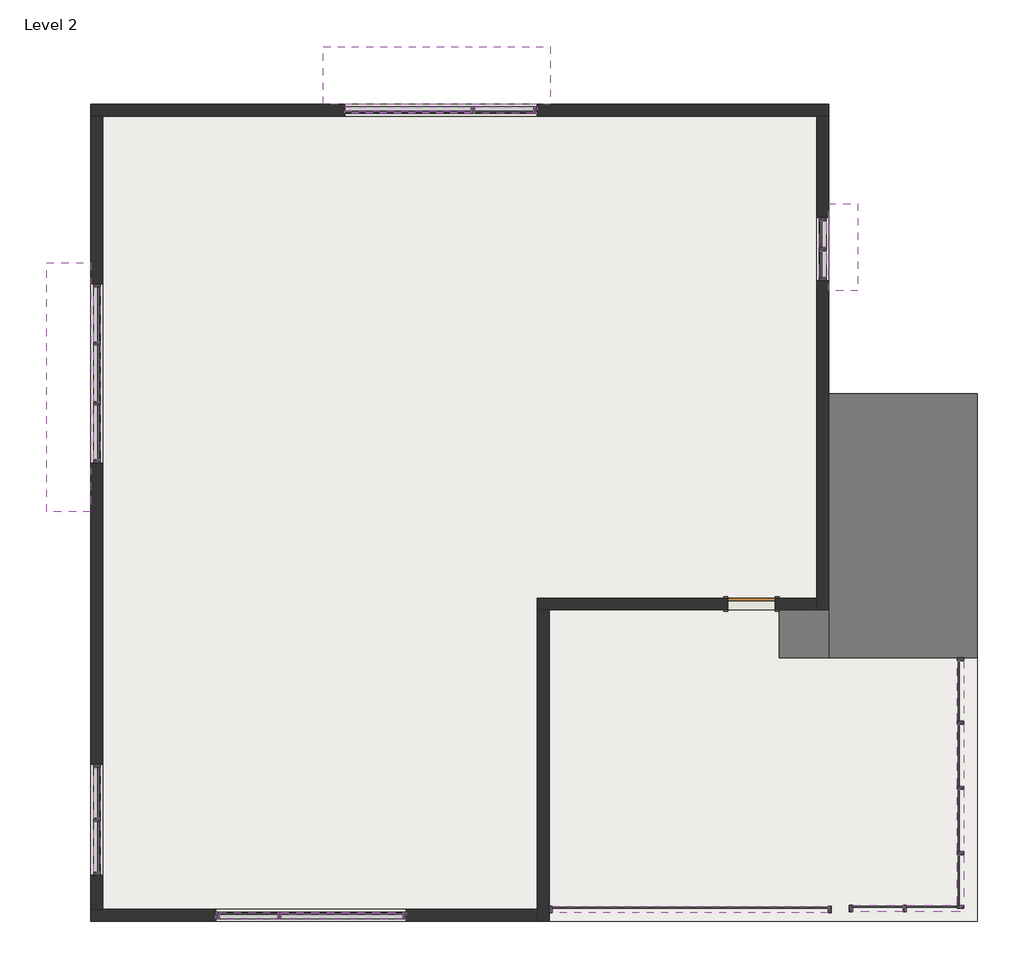
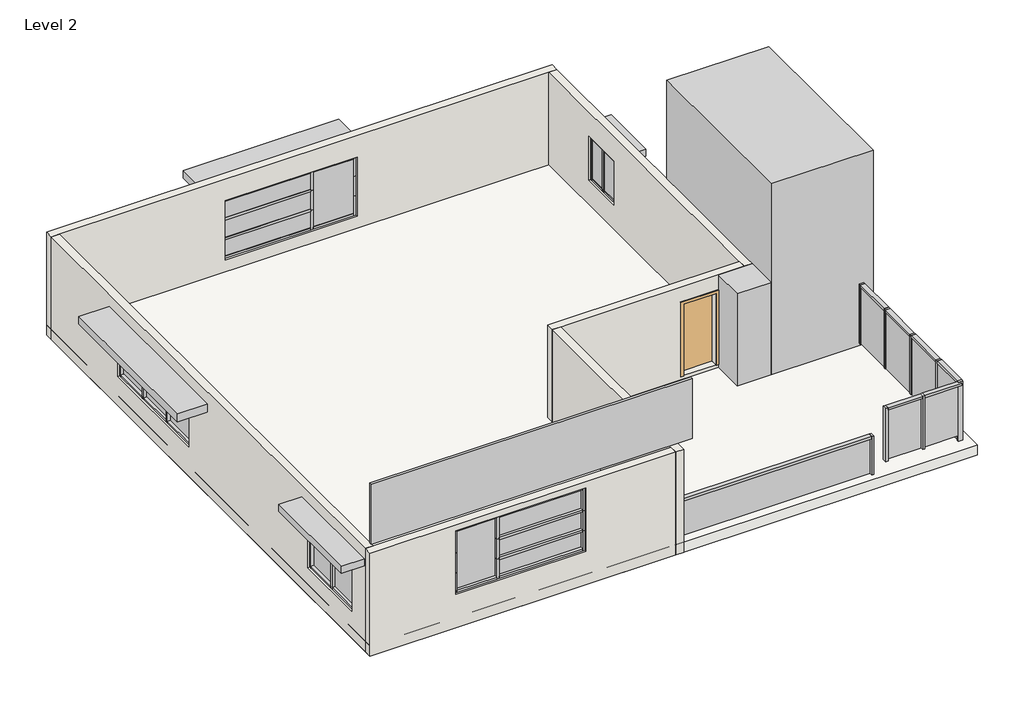
# One storey: 67 members, 22 plates, 6 walls, 4 proxies, 1 door, 1 roof.
"""IFC4 building model written with IfcOpenShell, lengths in millimetres."""

from ifc_helpers import new_model, si_unit, frame, origin, place, context, project, spatial, polyline, outline, extrude, faceted_brep, transform, mapped, element, save
from components import generic_models_10_generic_models_10_d4c633cf, generic_models_11_generic_models_11_9e8de572, generic_models_2_generic_models_2_10608999, generic_models_9_generic_models_9_222cebfa, door_0ca8825f, member_e6b9f524, member_eadc486f, member_9597caa3, member_f68a8c1e, member_c273ec95, member_b59b363a, member_48a7c542, member_a8f28920, member_ca95d35f, member_6d95fc69, member_971db604, member_6ef8dc49, member_801a2072, member_ed31d27a, member_2fbbe8c6, member_1434c356, member_89a24a7a, member_0b7646a3, member_9869c819, member_19a13f65, member_b030ebd8, member_54a35e60, member_39111128, member_6133cf7c, member_2569944f, member_814d5477, member_c450aece, member_9fa6ebbc, member_96c24052, member_491a8506, member_693a6220, system_panel_glazed_93d7cfd2, system_panel_glazed_c682d145, system_panel_glazed_b2f512c6, system_panel_glazed_6011e45a, system_panel_glazed_1356a548, system_panel_glazed_90125d95, system_panel_glazed_daa3f2c1, system_panel_glazed_8ae820b6, system_panel_glazed_a24099ce, system_panel_glazed_da159ad5, system_panel_glazed_d098f70f, system_panel_glazed_c8d94a63, system_panel_glazed_5b59eb94, system_panel_glazed_618c1181, system_panel_glazed_0e829309, system_panel_glazed_645b7f4f, system_panel_glazed_7de21dfc

model = new_model("IFC4")

# Units and contexts
model_context = context("Model", 3, world=origin())
ifc_project = project(units=[si_unit("LENGTHUNIT", "METRE", prefix="MILLI")], contexts=[model_context])

# Site, building, storey
site = spatial("IfcSite", under=ifc_project)
building = spatial("IfcBuilding", under=site)
storey = spatial("IfcBuildingStorey", under=building, Name="Level 2", Elevation=3048.0)

# Proxies
placement = place(None, origin())
generic_models_10_generic_models_10_shape = generic_models_10_generic_models_10_d4c633cf(model_context)
element("IfcBuildingElementProxy", 1, Name="Generic Models 10 : Generic Models 10", ObjectType="Generic Models 10 : Generic Models 10", at=placement, inside=storey, context=model_context, shape_type="MappedRepresentation", body=[
    mapped(generic_models_10_generic_models_10_shape, transform((0.0, 0.0, 0.0), x_axis=(1.0, 0.0, 0.0), y_axis=(0.0, 1.0, 0.0), z_axis=(0.0, 0.0, 1.0))),
])
generic_models_11_generic_models_11_shape = generic_models_11_generic_models_11_9e8de572(model_context)
element("IfcBuildingElementProxy", 2, Name="Generic Models 11 : Generic Models 11", ObjectType="Generic Models 11 : Generic Models 11", at=placement, inside=storey, context=model_context, shape_type="MappedRepresentation", body=[
    mapped(generic_models_11_generic_models_11_shape, transform((0.0, 0.0, 0.0), x_axis=(1.0, 0.0, 0.0), y_axis=(0.0, 1.0, 0.0), z_axis=(0.0, 0.0, 1.0))),
])
generic_models_2_generic_models_2_shape = generic_models_2_generic_models_2_10608999(model_context)
element("IfcBuildingElementProxy", 3, Name="Generic Models 2 : Generic Models 2", ObjectType="Generic Models 2 : Generic Models 2", at=placement, inside=storey, context=model_context, shape_type="MappedRepresentation", body=[
    mapped(generic_models_2_generic_models_2_shape, transform((0.0, 0.0, 0.0), x_axis=(1.0, 0.0, 0.0), y_axis=(0.0, 1.0, 0.0), z_axis=(0.0, 0.0, 1.0))),
])
generic_models_9_generic_models_9_shape = generic_models_9_generic_models_9_222cebfa(model_context)
element("IfcBuildingElementProxy", 4, Name="Generic Models 9 : Generic Models 9", ObjectType="Generic Models 9 : Generic Models 9", at=placement, inside=storey, context=model_context, shape_type="MappedRepresentation", body=[
    mapped(generic_models_9_generic_models_9_shape, transform((0.0, 0.0, 0.0), x_axis=(1.0, 0.0, 0.0), y_axis=(0.0, 1.0, 0.0), z_axis=(0.0, 0.0, 1.0))),
])

# Door
door_shape = door_0ca8825f(model_context)
element("IfcDoor", 5, ObjectType="Single-Flush : 36\" x 84\"", at=placement, inside=storey, context=model_context, shape_type="MappedRepresentation", body=[
    mapped(door_shape, transform((-7357.3120831, -6017.2945627, 3454.4), x_axis=(1.0, 0.0, 0.0), y_axis=(0.0, 1.0, 0.0), z_axis=(0.0, 0.0, 1.0))),
])

# Members
member_shape = member_e6b9f524(model_context)
element("IfcMember", 6, ObjectType="Rectangular Mullion : 2.5\" x 5\" rectangular", at=placement, inside=storey, context=model_context, shape_type="MappedRepresentation", body=[
    mapped(member_shape, transform((-16456.8620831, -11998.9945627, 5914.7350313), x_axis=(0.0, 0.0, 1.0), y_axis=(0.0, -1.0, 0.0), z_axis=(1.0, 0.0, 0.0))),
])
element("IfcMember", 7, ObjectType="Rectangular Mullion : 2.5\" x 5\" rectangular", at=placement, inside=storey, context=model_context, shape_type="MappedRepresentation", body=[
    mapped(member_shape, transform((-17580.8120831, -11998.9945627, 4036.0212725), x_axis=(0.0, 0.0, -1.0), y_axis=(0.0, -1.0, 0.0), z_axis=(-1.0, 0.0, 0.0))),
])
member_2_shape = member_eadc486f(model_context)
element("IfcMember", 8, ObjectType="Rectangular Mullion : 2.5\" x 5\" rectangular", at=placement, inside=storey, context=model_context, shape_type="MappedRepresentation", body=[
    mapped(member_2_shape, transform((-14050.2120831, -11998.9945627, 5914.7350313), x_axis=(0.0, 0.0, 1.0), y_axis=(0.0, -1.0, 0.0), z_axis=(1.0, 0.0, 0.0))),
])
element("IfcMember", 9, ObjectType="Rectangular Mullion : 2.5\" x 5\" rectangular", at=placement, inside=storey, context=model_context, shape_type="MappedRepresentation", body=[
    mapped(member_2_shape, transform((-16393.3620831, -11998.9945627, 4036.0212725), x_axis=(0.0, 0.0, -1.0), y_axis=(0.0, -1.0, 0.0), z_axis=(-1.0, 0.0, 0.0))),
])
member_3_shape = member_9597caa3(model_context)
element("IfcMember", 10, ObjectType="Rectangular Mullion : 2.5\" x 5\" rectangular", at=placement, inside=storey, context=model_context, shape_type="MappedRepresentation", body=[
    mapped(member_3_shape, transform((-14050.2120831, -11998.9945627, 5221.3329246), x_axis=(0.0, 0.0, 1.0), y_axis=(0.0, -1.0, 0.0), z_axis=(1.0, 0.0, 0.0))),
])
element("IfcMember", 11, ObjectType="Rectangular Mullion : 2.5\" x 5\" rectangular", at=placement, inside=storey, context=model_context, shape_type="MappedRepresentation", body=[
    mapped(member_3_shape, transform((-14050.2120831, -11998.9945627, 4628.6770985), x_axis=(0.0, 0.0, 1.0), y_axis=(0.0, -1.0, 0.0), z_axis=(1.0, 0.0, 0.0))),
])
member_4_shape = member_f68a8c1e(model_context)
element("IfcMember", 12, ObjectType="Rectangular Mullion : 2.5\" x 5\" rectangular", at=placement, inside=storey, context=model_context, shape_type="MappedRepresentation", body=[
    mapped(member_4_shape, transform((-17644.3120831, -11998.9945627, 5221.3329246), x_axis=(-1.0, 0.0, 0.0), y_axis=(0.0, -1.0, 0.0), z_axis=(0.0, 0.0, 1.0))),
])
element("IfcMember", 13, ObjectType="Rectangular Mullion : 2.5\" x 5\" rectangular", at=placement, inside=storey, context=model_context, shape_type="MappedRepresentation", body=[
    mapped(member_4_shape, transform((-17644.3120831, -11998.9945627, 4628.6770985), x_axis=(-1.0, 0.0, 0.0), y_axis=(0.0, -1.0, 0.0), z_axis=(0.0, 0.0, 1.0))),
])
member_5_shape = member_c273ec95(model_context)
element("IfcMember", 14, ObjectType="Rectangular Mullion : 2.5\" x 5\" rectangular", at=placement, inside=storey, context=model_context, shape_type="MappedRepresentation", body=[
    mapped(member_5_shape, transform((-16425.1120831, -11998.9945627, 4628.6770985), x_axis=(1.0, 0.0, 0.0), y_axis=(0.0, -1.0, 0.0), z_axis=(0.0, 0.0, -1.0))),
])
element("IfcMember", 15, ObjectType="Rectangular Mullion : 2.5\" x 5\" rectangular", at=placement, inside=storey, context=model_context, shape_type="MappedRepresentation", body=[
    mapped(member_5_shape, transform((-16425.1120831, -11998.9945627, 4036.0212725), x_axis=(1.0, 0.0, 0.0), y_axis=(0.0, -1.0, 0.0), z_axis=(0.0, 0.0, -1.0))),
])
element("IfcMember", 16, ObjectType="Rectangular Mullion : 2.5\" x 5\" rectangular", at=placement, inside=storey, context=model_context, shape_type="MappedRepresentation", body=[
    mapped(member_4_shape, transform((-13986.7120831, -11998.9945627, 4628.6770985), x_axis=(1.0, 0.0, 0.0), y_axis=(0.0, -1.0, 0.0), z_axis=(0.0, 0.0, -1.0))),
])
element("IfcMember", 17, ObjectType="Rectangular Mullion : 2.5\" x 5\" rectangular", at=placement, inside=storey, context=model_context, shape_type="MappedRepresentation", body=[
    mapped(member_4_shape, transform((-13986.7120831, -11998.9945627, 4036.0212725), x_axis=(1.0, 0.0, 0.0), y_axis=(0.0, -1.0, 0.0), z_axis=(0.0, 0.0, -1.0))),
])
member_6_shape = member_b59b363a(model_context)
element("IfcMember", 18, ObjectType="Rectangular Mullion : 2.5\" x 5\" rectangular", at=placement, inside=storey, context=model_context, shape_type="MappedRepresentation", body=[
    mapped(member_6_shape, transform((-16425.1120831, -11998.9945627, 5221.3329246), x_axis=(1.0, 0.0, 0.0), y_axis=(0.0, -1.0, 0.0), z_axis=(0.0, 0.0, -1.0))),
])
member_7_shape = member_48a7c542(model_context)
element("IfcMember", 19, ObjectType="Rectangular Mullion : 2.5\" x 5\" rectangular", at=placement, inside=storey, context=model_context, shape_type="MappedRepresentation", body=[
    mapped(member_7_shape, transform((-17644.3120831, -11998.9945627, 5914.7350313), x_axis=(-1.0, 0.0, 0.0), y_axis=(0.0, -1.0, 0.0), z_axis=(0.0, 0.0, 1.0))),
])
element("IfcMember", 20, ObjectType="Rectangular Mullion : 2.5\" x 5\" rectangular", at=placement, inside=storey, context=model_context, shape_type="MappedRepresentation", body=[
    mapped(member_7_shape, transform((-13986.7120831, -11998.9945627, 5221.3329246), x_axis=(1.0, 0.0, 0.0), y_axis=(0.0, -1.0, 0.0), z_axis=(0.0, 0.0, -1.0))),
])
member_8_shape = member_a8f28920(model_context)
element("IfcMember", 21, ObjectType="Rectangular Mullion : 2.5\" x 5\" rectangular", at=placement, inside=storey, context=model_context, shape_type="MappedRepresentation", body=[
    mapped(member_8_shape, transform((-11243.5120831, -11884.6945627, 4498.5631063), x_axis=(-1.0, 0.0, 0.0), y_axis=(0.0, -1.0, 0.0), z_axis=(0.0, 0.0, 1.0))),
])
member_9_shape = member_ca95d35f(model_context)
element("IfcMember", 22, ObjectType="Rectangular Mullion : 2.5\" x 5\" rectangular", at=placement, inside=storey, context=model_context, shape_type="MappedRepresentation", body=[
    mapped(member_9_shape, transform((-5884.1120831, -11884.6945627, 4498.5631063), x_axis=(0.0, 0.0, 1.0), y_axis=(0.0, -1.0, 0.0), z_axis=(1.0, 0.0, 0.0))),
])
element("IfcMember", 23, ObjectType="Rectangular Mullion : 2.5\" x 5\" rectangular", at=placement, inside=storey, context=model_context, shape_type="MappedRepresentation", body=[
    mapped(member_8_shape, transform((-5820.6120831, -11884.6945627, 3352.8), x_axis=(1.0, 0.0, 0.0), y_axis=(0.0, -1.0, 0.0), z_axis=(0.0, 0.0, -1.0))),
])
member_10_shape = member_6d95fc69(model_context)
element("IfcMember", 24, ObjectType="Rectangular Mullion : 2.5\" x 5\" rectangular", at=placement, inside=storey, context=model_context, shape_type="MappedRepresentation", body=[
    mapped(member_10_shape, transform((-3342.9519864, -11865.0422302, 5188.7151924), x_axis=(0.0, -1.0, 0.0), y_axis=(1.0, 0.0, 0.0), z_axis=(0.0, 0.0, 1.0))),
])
element("IfcMember", 25, ObjectType="Rectangular Mullion : 2.5\" x 5\" rectangular", at=placement, inside=storey, context=model_context, shape_type="MappedRepresentation", body=[
    mapped(member_10_shape, transform((-3342.9519864, -7045.9945627, 3433.2272233), x_axis=(0.0, 1.0, 0.0), y_axis=(1.0, 0.0, 0.0), z_axis=(0.0, 0.0, -1.0))),
])
member_11_shape = member_971db604(model_context)
element("IfcMember", 26, ObjectType="Rectangular Mullion : 2.5\" x 5\" rectangular", at=placement, inside=storey, context=model_context, shape_type="MappedRepresentation", body=[
    mapped(member_11_shape, transform((-5476.5519864, -11865.0422302, 5172.7154588), x_axis=(-1.0, 0.0, 0.0), y_axis=(0.0, -1.0, 0.0), z_axis=(0.0, 0.0, 1.0))),
])
member_12_shape = member_6ef8dc49(model_context)
element("IfcMember", 27, ObjectType="Rectangular Mullion : 2.5\" x 5\" rectangular", at=placement, inside=storey, context=model_context, shape_type="MappedRepresentation", body=[
    mapped(member_12_shape, transform((-3342.9519864, -11865.0422302, 5172.7154588), x_axis=(0.0, 0.0, 1.0), y_axis=(0.0, -1.0, 0.0), z_axis=(1.0, 0.0, 0.0))),
])
member_13_shape = member_801a2072(model_context)
element("IfcMember", 28, ObjectType="Rectangular Mullion : 2.5\" x 5\" rectangular", at=placement, inside=storey, context=model_context, shape_type="MappedRepresentation", body=[
    mapped(member_13_shape, transform((-3342.9519864, -10829.9922302, 5188.7151924), x_axis=(0.0, 0.0, 1.0), y_axis=(1.0, 0.0, 0.0), z_axis=(0.0, 1.0, 0.0))),
])
element("IfcMember", 29, ObjectType="Rectangular Mullion : 2.5\" x 5\" rectangular", at=placement, inside=storey, context=model_context, shape_type="MappedRepresentation", body=[
    mapped(member_13_shape, transform((-4441.5019864, -11865.0422302, 5172.7154588), x_axis=(0.0, 0.0, 1.0), y_axis=(0.0, -1.0, 0.0), z_axis=(1.0, 0.0, 0.0))),
])
element("IfcMember", 30, ObjectType="Rectangular Mullion : 2.5\" x 5\" rectangular", at=placement, inside=storey, context=model_context, shape_type="MappedRepresentation", body=[
    mapped(member_13_shape, transform((-19930.3120831, -10133.8038033, 5567.4357586), x_axis=(0.0, 0.0, 1.0), y_axis=(-1.0, 0.0, 0.0), z_axis=(0.0, -1.0, 0.0))),
])
element("IfcMember", 31, ObjectType="Rectangular Mullion : 2.5\" x 5\" rectangular", at=placement, inside=storey, context=model_context, shape_type="MappedRepresentation", body=[
    mapped(member_13_shape, transform((-19930.3120831, -11168.8538033, 5567.4357586), x_axis=(0.0, 0.0, 1.0), y_axis=(-1.0, 0.0, 0.0), z_axis=(0.0, -1.0, 0.0))),
])
member_14_shape = member_ed31d27a(model_context)
element("IfcMember", 32, ObjectType="Rectangular Mullion : 2.5\" x 5\" rectangular", at=placement, inside=storey, context=model_context, shape_type="MappedRepresentation", body=[
    mapped(member_14_shape, transform((-4409.7519864, -11865.0422302, 3593.4675285), x_axis=(1.0, 0.0, 0.0), y_axis=(0.0, -1.0, 0.0), z_axis=(0.0, 0.0, -1.0))),
])
member_15_shape = member_2fbbe8c6(model_context)
element("IfcMember", 33, ObjectType="Rectangular Mullion : 2.5\" x 5\" rectangular", at=placement, inside=storey, context=model_context, shape_type="MappedRepresentation", body=[
    mapped(member_15_shape, transform((-3342.9519864, -10798.2422302, 3433.2272233), x_axis=(0.0, 1.0, 0.0), y_axis=(1.0, 0.0, 0.0), z_axis=(0.0, 0.0, -1.0))),
])
element("IfcMember", 34, ObjectType="Rectangular Mullion : 2.5\" x 5\" rectangular", at=placement, inside=storey, context=model_context, shape_type="MappedRepresentation", body=[
    mapped(member_15_shape, transform((-3342.9519864, -9547.4930077, 3433.2272233), x_axis=(0.0, 1.0, 0.0), y_axis=(1.0, 0.0, 0.0), z_axis=(0.0, 0.0, -1.0))),
])
element("IfcMember", 35, ObjectType="Rectangular Mullion : 2.5\" x 5\" rectangular", at=placement, inside=storey, context=model_context, shape_type="MappedRepresentation", body=[
    mapped(member_15_shape, transform((-3342.9519864, -8296.7437852, 3433.2272233), x_axis=(0.0, 1.0, 0.0), y_axis=(1.0, 0.0, 0.0), z_axis=(0.0, 0.0, -1.0))),
])
member_16_shape = member_1434c356(model_context)
element("IfcMember", 36, ObjectType="Rectangular Mullion : 2.5\" x 5\" rectangular", at=placement, inside=storey, context=model_context, shape_type="MappedRepresentation", body=[
    mapped(member_16_shape, transform((-3342.9519864, -9579.2430077, 5188.7151924), x_axis=(0.0, 0.0, 1.0), y_axis=(1.0, 0.0, 0.0), z_axis=(0.0, 1.0, 0.0))),
])
element("IfcMember", 37, ObjectType="Rectangular Mullion : 2.5\" x 5\" rectangular", at=placement, inside=storey, context=model_context, shape_type="MappedRepresentation", body=[
    mapped(member_16_shape, transform((-3342.9519864, -8328.4937852, 5188.7151924), x_axis=(0.0, 0.0, 1.0), y_axis=(1.0, 0.0, 0.0), z_axis=(0.0, 1.0, 0.0))),
])
member_17_shape = member_89a24a7a(model_context)
element("IfcMember", 38, ObjectType="Rectangular Mullion : 2.5\" x 5\" rectangular", at=placement, inside=storey, context=model_context, shape_type="MappedRepresentation", body=[
    mapped(member_17_shape, transform((-3342.9519864, -7109.4945627, 5188.7151924), x_axis=(0.0, 0.0, 1.0), y_axis=(1.0, 0.0, 0.0), z_axis=(0.0, 1.0, 0.0))),
])
member_18_shape = member_0b7646a3(model_context)
element("IfcMember", 39, ObjectType="Rectangular Mullion : 2.5\" x 5\" rectangular", at=placement, inside=storey, context=model_context, shape_type="MappedRepresentation", body=[
    mapped(member_18_shape, transform((-5985.7120831, 834.3554373, 4074.9957322), x_axis=(0.0, 0.0, -1.0), y_axis=(1.0, 0.0, 0.0), z_axis=(0.0, -1.0, 0.0))),
])
element("IfcMember", 40, ObjectType="Rectangular Mullion : 2.5\" x 5\" rectangular", at=placement, inside=storey, context=model_context, shape_type="MappedRepresentation", body=[
    mapped(member_18_shape, transform((-5985.7120831, 256.5054373, 4074.9957322), x_axis=(0.0, 0.0, -1.0), y_axis=(1.0, 0.0, 0.0), z_axis=(0.0, -1.0, 0.0))),
])
member_19_shape = member_9869c819(model_context)
element("IfcMember", 41, ObjectType="Rectangular Mullion : 2.5\" x 5\" rectangular", at=placement, inside=storey, context=model_context, shape_type="MappedRepresentation", body=[
    mapped(member_19_shape, transform((-5985.7120831, 802.6054373, 4074.9957322), x_axis=(0.0, 1.0, 0.0), y_axis=(1.0, 0.0, 0.0), z_axis=(0.0, 0.0, -1.0))),
])
element("IfcMember", 42, ObjectType="Rectangular Mullion : 2.5\" x 5\" rectangular", at=placement, inside=storey, context=model_context, shape_type="MappedRepresentation", body=[
    mapped(member_18_shape, transform((-5985.7120831, 770.8554373, 5376.6144653), x_axis=(0.0, 0.0, 1.0), y_axis=(1.0, 0.0, 0.0), z_axis=(0.0, 1.0, 0.0))),
])
element("IfcMember", 43, ObjectType="Rectangular Mullion : 2.5\" x 5\" rectangular", at=placement, inside=storey, context=model_context, shape_type="MappedRepresentation", body=[
    mapped(member_18_shape, transform((-5985.7120831, 1348.7054373, 5376.6144653), x_axis=(0.0, 0.0, 1.0), y_axis=(1.0, 0.0, 0.0), z_axis=(0.0, 1.0, 0.0))),
])
member_20_shape = member_19a13f65(model_context)
element("IfcMember", 44, ObjectType="Rectangular Mullion : 2.5\" x 5\" rectangular", at=placement, inside=storey, context=model_context, shape_type="MappedRepresentation", body=[
    mapped(member_20_shape, transform((-5985.7120831, 193.0054373, 5376.6144653), x_axis=(0.0, -1.0, 0.0), y_axis=(1.0, 0.0, 0.0), z_axis=(0.0, 0.0, 1.0))),
])
element("IfcMember", 45, ObjectType="Rectangular Mullion : 2.5\" x 5\" rectangular", at=placement, inside=storey, context=model_context, shape_type="MappedRepresentation", body=[
    mapped(member_20_shape, transform((-5985.7120831, 1412.2054373, 4074.9957322), x_axis=(0.0, 1.0, 0.0), y_axis=(1.0, 0.0, 0.0), z_axis=(0.0, 0.0, -1.0))),
])
member_21_shape = member_b030ebd8(model_context)
element("IfcMember", 46, ObjectType="Rectangular Mullion : 2.5\" x 5\" rectangular", at=placement, inside=storey, context=model_context, shape_type="MappedRepresentation", body=[
    mapped(member_21_shape, transform((-15167.8120831, 3469.6054373, 5462.9315541), x_axis=(0.0, 0.0, 1.0), y_axis=(0.0, 1.0, 0.0), z_axis=(-1.0, 0.0, 0.0))),
])
member_22_shape = member_54a35e60(model_context)
element("IfcMember", 47, ObjectType="Rectangular Mullion : 2.5\" x 5\" rectangular", at=placement, inside=storey, context=model_context, shape_type="MappedRepresentation", body=[
    mapped(member_22_shape, transform((-12672.2620831, 3469.6054373, 5462.9315541), x_axis=(0.0, 0.0, 1.0), y_axis=(0.0, 1.0, 0.0), z_axis=(-1.0, 0.0, 0.0))),
])
member_23_shape = member_39111128(model_context)
element("IfcMember", 48, ObjectType="Rectangular Mullion : 2.5\" x 5\" rectangular", at=placement, inside=storey, context=model_context, shape_type="MappedRepresentation", body=[
    mapped(member_23_shape, transform((-11472.1120831, 3469.6054373, 4878.7141783), x_axis=(1.0, 0.0, 0.0), y_axis=(0.0, 1.0, 0.0), z_axis=(0.0, 0.0, 1.0))),
])
element("IfcMember", 49, ObjectType="Rectangular Mullion : 2.5\" x 5\" rectangular", at=placement, inside=storey, context=model_context, shape_type="MappedRepresentation", body=[
    mapped(member_23_shape, transform((-11472.1120831, 3469.6054373, 5462.9315541), x_axis=(1.0, 0.0, 0.0), y_axis=(0.0, 1.0, 0.0), z_axis=(0.0, 0.0, 1.0))),
])
element("IfcMember", 50, ObjectType="Rectangular Mullion : 2.5\" x 5\" rectangular", at=placement, inside=storey, context=model_context, shape_type="MappedRepresentation", body=[
    mapped(member_21_shape, transform((-12735.7620831, 3469.6054373, 3710.2794265), x_axis=(0.0, 0.0, -1.0), y_axis=(0.0, 1.0, 0.0), z_axis=(1.0, 0.0, 0.0))),
])
element("IfcMember", 51, ObjectType="Rectangular Mullion : 2.5\" x 5\" rectangular", at=placement, inside=storey, context=model_context, shape_type="MappedRepresentation", body=[
    mapped(member_22_shape, transform((-11535.6120831, 3469.6054373, 3710.2794265), x_axis=(0.0, 0.0, -1.0), y_axis=(0.0, 1.0, 0.0), z_axis=(1.0, 0.0, 0.0))),
])
element("IfcMember", 52, ObjectType="Rectangular Mullion : 2.5\" x 5\" rectangular", at=placement, inside=storey, context=model_context, shape_type="MappedRepresentation", body=[
    mapped(member_23_shape, transform((-11472.1120831, 3469.6054373, 4294.4968024), x_axis=(1.0, 0.0, 0.0), y_axis=(0.0, 1.0, 0.0), z_axis=(0.0, 0.0, 1.0))),
])
member_24_shape = member_6133cf7c(model_context)
element("IfcMember", 53, ObjectType="Rectangular Mullion : 2.5\" x 5\" rectangular", at=placement, inside=storey, context=model_context, shape_type="MappedRepresentation", body=[
    mapped(member_24_shape, transform((-12704.0120831, 3469.6054373, 3710.2794265), x_axis=(-1.0, 0.0, 0.0), y_axis=(0.0, 1.0, 0.0), z_axis=(0.0, 0.0, -1.0))),
])
member_25_shape = member_2569944f(model_context)
element("IfcMember", 54, ObjectType="Rectangular Mullion : 2.5\" x 5\" rectangular", at=placement, inside=storey, context=model_context, shape_type="MappedRepresentation", body=[
    mapped(member_25_shape, transform((-15167.8120831, 3469.6054373, 4294.4968024), x_axis=(0.0, 0.0, 1.0), y_axis=(0.0, 1.0, 0.0), z_axis=(-1.0, 0.0, 0.0))),
])
element("IfcMember", 55, ObjectType="Rectangular Mullion : 2.5\" x 5\" rectangular", at=placement, inside=storey, context=model_context, shape_type="MappedRepresentation", body=[
    mapped(member_25_shape, transform((-15167.8120831, 3469.6054373, 4878.7141783), x_axis=(0.0, 0.0, 1.0), y_axis=(0.0, 1.0, 0.0), z_axis=(-1.0, 0.0, 0.0))),
])
element("IfcMember", 56, ObjectType="Rectangular Mullion : 2.5\" x 5\" rectangular", at=placement, inside=storey, context=model_context, shape_type="MappedRepresentation", body=[
    mapped(member_24_shape, transform((-12704.0120831, 3469.6054373, 4294.4968024), x_axis=(-1.0, 0.0, 0.0), y_axis=(0.0, 1.0, 0.0), z_axis=(0.0, 0.0, -1.0))),
])
element("IfcMember", 57, ObjectType="Rectangular Mullion : 2.5\" x 5\" rectangular", at=placement, inside=storey, context=model_context, shape_type="MappedRepresentation", body=[
    mapped(member_24_shape, transform((-12704.0120831, 3469.6054373, 4878.7141783), x_axis=(-1.0, 0.0, 0.0), y_axis=(0.0, 1.0, 0.0), z_axis=(0.0, 0.0, -1.0))),
])
member_26_shape = member_814d5477(model_context)
element("IfcMember", 58, ObjectType="Rectangular Mullion : 2.5\" x 5\" rectangular", at=placement, inside=storey, context=model_context, shape_type="MappedRepresentation", body=[
    mapped(member_26_shape, transform((-19930.3120831, -10165.5538033, 3840.6220219), x_axis=(0.0, -1.0, 0.0), y_axis=(-1.0, 0.0, 0.0), z_axis=(0.0, 0.0, -1.0))),
])
element("IfcMember", 59, ObjectType="Rectangular Mullion : 2.5\" x 5\" rectangular", at=placement, inside=storey, context=model_context, shape_type="MappedRepresentation", body=[
    mapped(member_13_shape, transform((-19930.3120831, -10197.3038033, 3840.6220219), x_axis=(0.0, 0.0, -1.0), y_axis=(-1.0, 0.0, 0.0), z_axis=(0.0, 1.0, 0.0))),
])
element("IfcMember", 60, ObjectType="Rectangular Mullion : 2.5\" x 5\" rectangular", at=placement, inside=storey, context=model_context, shape_type="MappedRepresentation", body=[
    mapped(member_13_shape, transform((-19930.3120831, -9162.2538033, 3840.6220219), x_axis=(0.0, 0.0, -1.0), y_axis=(-1.0, 0.0, 0.0), z_axis=(0.0, 1.0, 0.0))),
])
member_27_shape = member_c450aece(model_context)
element("IfcMember", 61, ObjectType="Rectangular Mullion : 2.5\" x 5\" rectangular", at=placement, inside=storey, context=model_context, shape_type="MappedRepresentation", body=[
    mapped(member_27_shape, transform((-19930.3120831, -11232.3538033, 3840.6220219), x_axis=(0.0, -1.0, 0.0), y_axis=(-1.0, 0.0, 0.0), z_axis=(0.0, 0.0, -1.0))),
])
element("IfcMember", 62, ObjectType="Rectangular Mullion : 2.5\" x 5\" rectangular", at=placement, inside=storey, context=model_context, shape_type="MappedRepresentation", body=[
    mapped(member_27_shape, transform((-19930.3120831, -9098.7538033, 5567.4357586), x_axis=(0.0, 1.0, 0.0), y_axis=(-1.0, 0.0, 0.0), z_axis=(0.0, 0.0, 1.0))),
])
member_28_shape = member_9fa6ebbc(model_context)
element("IfcMember", 63, ObjectType="Rectangular Mullion : 2.5\" x 5\" rectangular", at=placement, inside=storey, context=model_context, shape_type="MappedRepresentation", body=[
    mapped(member_28_shape, transform((-19930.3120831, -2196.2572471, 3916.4749442), x_axis=(0.0, 0.0, -1.0), y_axis=(-1.0, 0.0, 0.0), z_axis=(0.0, 1.0, 0.0))),
])
element("IfcMember", 64, ObjectType="Rectangular Mullion : 2.5\" x 5\" rectangular", at=placement, inside=storey, context=model_context, shape_type="MappedRepresentation", body=[
    mapped(member_28_shape, transform((-19930.3120831, 67.3673842, 3916.4749442), x_axis=(0.0, 0.0, -1.0), y_axis=(-1.0, 0.0, 0.0), z_axis=(0.0, 1.0, 0.0))),
])
member_29_shape = member_96c24052(model_context)
element("IfcMember", 65, ObjectType="Rectangular Mullion : 2.5\" x 5\" rectangular", at=placement, inside=storey, context=model_context, shape_type="MappedRepresentation", body=[
    mapped(member_29_shape, transform((-19930.3120831, -1048.5699315, 3916.4749442), x_axis=(0.0, 0.0, -1.0), y_axis=(-1.0, 0.0, 0.0), z_axis=(0.0, 1.0, 0.0))),
])
member_30_shape = member_491a8506(model_context)
element("IfcMember", 66, ObjectType="Rectangular Mullion : 2.5\" x 5\" rectangular", at=placement, inside=storey, context=model_context, shape_type="MappedRepresentation", body=[
    mapped(member_30_shape, transform((-19930.3120831, -2164.5072471, 3916.4749442), x_axis=(0.0, -1.0, 0.0), y_axis=(-1.0, 0.0, 0.0), z_axis=(0.0, 0.0, -1.0))),
])
element("IfcMember", 67, ObjectType="Rectangular Mullion : 2.5\" x 5\" rectangular", at=placement, inside=storey, context=model_context, shape_type="MappedRepresentation", body=[
    mapped(member_30_shape, transform((-19930.3120831, -1016.8199315, 3916.4749442), x_axis=(0.0, -1.0, 0.0), y_axis=(-1.0, 0.0, 0.0), z_axis=(0.0, 0.0, -1.0))),
])
element("IfcMember", 68, ObjectType="Rectangular Mullion : 2.5\" x 5\" rectangular", at=placement, inside=storey, context=model_context, shape_type="MappedRepresentation", body=[
    mapped(member_29_shape, transform((-19930.3120831, -2132.7572471, 5519.0574769), x_axis=(0.0, 0.0, 1.0), y_axis=(-1.0, 0.0, 0.0), z_axis=(0.0, -1.0, 0.0))),
])
element("IfcMember", 69, ObjectType="Rectangular Mullion : 2.5\" x 5\" rectangular", at=placement, inside=storey, context=model_context, shape_type="MappedRepresentation", body=[
    mapped(member_28_shape, transform((-19930.3120831, -985.0699315, 5519.0574769), x_axis=(0.0, 0.0, 1.0), y_axis=(-1.0, 0.0, 0.0), z_axis=(0.0, -1.0, 0.0))),
])
element("IfcMember", 70, ObjectType="Rectangular Mullion : 2.5\" x 5\" rectangular", at=placement, inside=storey, context=model_context, shape_type="MappedRepresentation", body=[
    mapped(member_28_shape, transform((-19930.3120831, -3248.6945627, 5519.0574769), x_axis=(0.0, 0.0, 1.0), y_axis=(-1.0, 0.0, 0.0), z_axis=(0.0, -1.0, 0.0))),
])
member_31_shape = member_693a6220(model_context)
element("IfcMember", 71, ObjectType="Rectangular Mullion : 2.5\" x 5\" rectangular", at=placement, inside=storey, context=model_context, shape_type="MappedRepresentation", body=[
    mapped(member_31_shape, transform((-19930.3120831, -3312.1945627, 3916.4749442), x_axis=(0.0, -1.0, 0.0), y_axis=(-1.0, 0.0, 0.0), z_axis=(0.0, 0.0, -1.0))),
])
element("IfcMember", 72, ObjectType="Rectangular Mullion : 2.5\" x 5\" rectangular", at=placement, inside=storey, context=model_context, shape_type="MappedRepresentation", body=[
    mapped(member_31_shape, transform((-19930.3120831, 130.8673842, 5519.0574769), x_axis=(0.0, 1.0, 0.0), y_axis=(-1.0, 0.0, 0.0), z_axis=(0.0, 0.0, 1.0))),
])

# Plates
system_panel_glazed_shape = system_panel_glazed_93d7cfd2(model_context)
element("IfcPlate", 73, ObjectType="System Panel : Glazed", at=placement, inside=storey, context=model_context, shape_type="MappedRepresentation", body=[
    mapped(system_panel_glazed_shape, transform((-15221.7870831, -11998.9945627, 4099.5212725), x_axis=(1.0, 0.0, 0.0), y_axis=(0.0, 1.0, 0.0), z_axis=(0.0, 0.0, 1.0))),
])
system_panel_glazed_2_shape = system_panel_glazed_c682d145(model_context)
element("IfcPlate", 74, ObjectType="System Panel : Glazed", at=placement, inside=storey, context=model_context, shape_type="MappedRepresentation", body=[
    mapped(system_panel_glazed_2_shape, transform((-15221.7870831, -11998.9945627, 4660.4270985), x_axis=(1.0, 0.0, 0.0), y_axis=(0.0, 1.0, 0.0), z_axis=(0.0, 0.0, 1.0))),
])
system_panel_glazed_3_shape = system_panel_glazed_b2f512c6(model_context)
element("IfcPlate", 75, ObjectType="System Panel : Glazed", at=placement, inside=storey, context=model_context, shape_type="MappedRepresentation", body=[
    mapped(system_panel_glazed_3_shape, transform((-17018.8370831, -11998.9945627, 4099.5212725), x_axis=(1.0, 0.0, 0.0), y_axis=(0.0, 1.0, 0.0), z_axis=(0.0, 0.0, 1.0))),
])
system_panel_glazed_4_shape = system_panel_glazed_6011e45a(model_context)
element("IfcPlate", 76, ObjectType="System Panel : Glazed", at=placement, inside=storey, context=model_context, shape_type="MappedRepresentation", body=[
    mapped(system_panel_glazed_4_shape, transform((-15221.7870831, -11998.9945627, 5253.0829246), x_axis=(1.0, 0.0, 0.0), y_axis=(0.0, 1.0, 0.0), z_axis=(0.0, 0.0, 1.0))),
])
system_panel_glazed_5_shape = system_panel_glazed_1356a548(model_context)
element("IfcPlate", 77, ObjectType="System Panel : Glazed", at=placement, inside=storey, context=model_context, shape_type="MappedRepresentation", body=[
    mapped(system_panel_glazed_5_shape, transform((-8532.0620831, -11884.6945627, 3352.8), x_axis=(1.0, 0.0, 0.0), y_axis=(0.0, 1.0, 0.0), z_axis=(0.0, 0.0, 1.0))),
])
system_panel_glazed_6_shape = system_panel_glazed_90125d95(model_context)
element("IfcPlate", 78, ObjectType="System Panel : Glazed", at=placement, inside=storey, context=model_context, shape_type="MappedRepresentation", body=[
    mapped(system_panel_glazed_6_shape, transform((-3342.9519864, -10172.8676189, 3433.2272233), x_axis=(0.0, 1.0, 0.0), y_axis=(-1.0, 0.0, 0.0), z_axis=(0.0, 0.0, 1.0))),
])
element("IfcPlate", 79, ObjectType="System Panel : Glazed", at=placement, inside=storey, context=model_context, shape_type="MappedRepresentation", body=[
    mapped(system_panel_glazed_6_shape, transform((-3342.9519864, -8922.1183964, 3433.2272233), x_axis=(0.0, 1.0, 0.0), y_axis=(-1.0, 0.0, 0.0), z_axis=(0.0, 0.0, 1.0))),
])
system_panel_glazed_7_shape = system_panel_glazed_daa3f2c1(model_context)
element("IfcPlate", 80, ObjectType="System Panel : Glazed", at=placement, inside=storey, context=model_context, shape_type="MappedRepresentation", body=[
    mapped(system_panel_glazed_7_shape, transform((-4927.2769864, -11865.0422302, 3593.4675285), x_axis=(1.0, 0.0, 0.0), y_axis=(0.0, 1.0, 0.0), z_axis=(0.0, 0.0, 1.0))),
])
system_panel_glazed_8_shape = system_panel_glazed_8ae820b6(model_context)
element("IfcPlate", 81, ObjectType="System Panel : Glazed", at=placement, inside=storey, context=model_context, shape_type="MappedRepresentation", body=[
    mapped(system_panel_glazed_8_shape, transform((-3860.4769864, -11865.0422302, 3593.4675285), x_axis=(1.0, 0.0, 0.0), y_axis=(0.0, 1.0, 0.0), z_axis=(0.0, 0.0, 1.0))),
])
system_panel_glazed_9_shape = system_panel_glazed_a24099ce(model_context)
element("IfcPlate", 82, ObjectType="System Panel : Glazed", at=placement, inside=storey, context=model_context, shape_type="MappedRepresentation", body=[
    mapped(system_panel_glazed_9_shape, transform((-3342.9519864, -11315.7672302, 3433.2272233), x_axis=(0.0, 1.0, 0.0), y_axis=(-1.0, 0.0, 0.0), z_axis=(0.0, 0.0, 1.0))),
])
system_panel_glazed_10_shape = system_panel_glazed_da159ad5(model_context)
element("IfcPlate", 83, ObjectType="System Panel : Glazed", at=placement, inside=storey, context=model_context, shape_type="MappedRepresentation", body=[
    mapped(system_panel_glazed_10_shape, transform((-3342.9519864, -7687.2441739, 3433.2272233), x_axis=(0.0, 1.0, 0.0), y_axis=(-1.0, 0.0, 0.0), z_axis=(0.0, 0.0, 1.0))),
])
system_panel_glazed_11_shape = system_panel_glazed_d098f70f(model_context)
element("IfcPlate", 84, ObjectType="System Panel : Glazed", at=placement, inside=storey, context=model_context, shape_type="MappedRepresentation", body=[
    mapped(system_panel_glazed_11_shape, transform((-5985.7120831, 513.6804373, 4138.4957322), x_axis=(0.0, 1.0, 0.0), y_axis=(-1.0, 0.0, 0.0), z_axis=(0.0, 0.0, 1.0))),
])
element("IfcPlate", 85, ObjectType="System Panel : Glazed", at=placement, inside=storey, context=model_context, shape_type="MappedRepresentation", body=[
    mapped(system_panel_glazed_11_shape, transform((-5985.7120831, 1091.5304373, 4138.4957322), x_axis=(0.0, 1.0, 0.0), y_axis=(-1.0, 0.0, 0.0), z_axis=(0.0, 0.0, 1.0))),
])
system_panel_glazed_12_shape = system_panel_glazed_c8d94a63(model_context)
element("IfcPlate", 86, ObjectType="System Panel : Glazed", at=placement, inside=storey, context=model_context, shape_type="MappedRepresentation", body=[
    mapped(system_panel_glazed_12_shape, transform((-13951.7870831, 3469.6054373, 4326.2468024), x_axis=(-1.0, 0.0, 0.0), y_axis=(0.0, -1.0, 0.0), z_axis=(0.0, 0.0, 1.0))),
])
system_panel_glazed_13_shape = system_panel_glazed_5b59eb94(model_context)
element("IfcPlate", 87, ObjectType="System Panel : Glazed", at=placement, inside=storey, context=model_context, shape_type="MappedRepresentation", body=[
    mapped(system_panel_glazed_13_shape, transform((-12103.9370831, 3469.6054373, 3773.7794265), x_axis=(-1.0, 0.0, 0.0), y_axis=(0.0, -1.0, 0.0), z_axis=(0.0, 0.0, 1.0))),
])
system_panel_glazed_14_shape = system_panel_glazed_618c1181(model_context)
element("IfcPlate", 88, ObjectType="System Panel : Glazed", at=placement, inside=storey, context=model_context, shape_type="MappedRepresentation", body=[
    mapped(system_panel_glazed_14_shape, transform((-13951.7870831, 3469.6054373, 3773.7794265), x_axis=(-1.0, 0.0, 0.0), y_axis=(0.0, -1.0, 0.0), z_axis=(0.0, 0.0, 1.0))),
])
element("IfcPlate", 89, ObjectType="System Panel : Glazed", at=placement, inside=storey, context=model_context, shape_type="MappedRepresentation", body=[
    mapped(system_panel_glazed_14_shape, transform((-13951.7870831, 3469.6054373, 4910.4641783), x_axis=(-1.0, 0.0, 0.0), y_axis=(0.0, -1.0, 0.0), z_axis=(0.0, 0.0, 1.0))),
])
system_panel_glazed_15_shape = system_panel_glazed_0e829309(model_context)
element("IfcPlate", 90, ObjectType="System Panel : Glazed", at=placement, inside=storey, context=model_context, shape_type="MappedRepresentation", body=[
    mapped(system_panel_glazed_15_shape, transform((-19930.3120831, -9648.0288033, 3904.1220219), x_axis=(0.0, -1.0, 0.0), y_axis=(1.0, 0.0, 0.0), z_axis=(0.0, 0.0, 1.0))),
])
element("IfcPlate", 91, ObjectType="System Panel : Glazed", at=placement, inside=storey, context=model_context, shape_type="MappedRepresentation", body=[
    mapped(system_panel_glazed_15_shape, transform((-19930.3120831, -10683.0788033, 3904.1220219), x_axis=(0.0, -1.0, 0.0), y_axis=(1.0, 0.0, 0.0), z_axis=(0.0, 0.0, 1.0))),
])
system_panel_glazed_16_shape = system_panel_glazed_645b7f4f(model_context)
element("IfcPlate", 92, ObjectType="System Panel : Glazed", at=placement, inside=storey, context=model_context, shape_type="MappedRepresentation", body=[
    mapped(system_panel_glazed_16_shape, transform((-19930.3120831, -458.8512736, 3979.9749442), x_axis=(0.0, -1.0, 0.0), y_axis=(1.0, 0.0, 0.0), z_axis=(0.0, 0.0, 1.0))),
])
element("IfcPlate", 93, ObjectType="System Panel : Glazed", at=placement, inside=storey, context=model_context, shape_type="MappedRepresentation", body=[
    mapped(system_panel_glazed_16_shape, transform((-19930.3120831, -2722.4759049, 3979.9749442), x_axis=(0.0, -1.0, 0.0), y_axis=(1.0, 0.0, 0.0), z_axis=(0.0, 0.0, 1.0))),
])
system_panel_glazed_17_shape = system_panel_glazed_7de21dfc(model_context)
element("IfcPlate", 94, ObjectType="System Panel : Glazed", at=placement, inside=storey, context=model_context, shape_type="MappedRepresentation", body=[
    mapped(system_panel_glazed_17_shape, transform((-19930.3120831, -1590.6635893, 3979.9749442), x_axis=(0.0, -1.0, 0.0), y_axis=(1.0, 0.0, 0.0), z_axis=(0.0, 0.0, 1.0))),
])

# Roof
element("IfcRoof", 95, ObjectType="Generic - 12\"", at=placement, inside=storey, context=model_context, shape_type="SweptSolid", body=[
    extrude(outline(polyline([(-20044.6120831, 3583.9054373), (-5871.4120831, 3583.9054373), (-5871.4120831, -1978.6945627), (-3013.9120831, -1978.6945627), (-3013.9120831, -12113.2945627), (-20044.6120831, -12113.2945627), (-20044.6120831, 3583.9054373)])), frame((0.0, 0.0, 3048.0), z_axis=(0.0, 0.0, 1.0), x_axis=(1.0, 0.0, 0.0)), (0.0, 0.0, 1.0), 304.8),
])

# Walls
element("IfcWall", 96, ObjectType="9\"", at=placement, inside=storey, context=model_context, shape_type="Brep", body=[
    faceted_brep([(-20044.6120831, 3355.3054373, 3048.0), (-19816.0120831, 3355.3054373, 3048.0), (-6100.0120831, 3355.3054373, 3048.0), (-5871.4120831, 3355.3054373, 3048.0), (-5871.4120831, 3355.3054373, 6096.0), (-6100.0120831, 3355.3054373, 6096.0), (-19816.0120831, 3355.3054373, 6096.0), (-20044.6120831, 3355.3054373, 6096.0), (-11472.1120831, 3355.3054373, 5462.9315541), (-11472.1120831, 3355.3054373, 3710.2794265), (-15167.8120831, 3355.3054373, 3710.2794265), (-15167.8120831, 3355.3054373, 5462.9315541), (-5871.4120831, 3583.9054373, 3048.0), (-20044.6120831, 3583.9054373, 3048.0), (-20044.6120831, 3583.9054373, 6096.0), (-5871.4120831, 3583.9054373, 6096.0), (-11472.1120831, 3583.9054373, 3710.2794265), (-11472.1120831, 3583.9054373, 5462.9315541), (-15167.8120831, 3583.9054373, 5462.9315541), (-15167.8120831, 3583.9054373, 3710.2794265)], [[[0, 1, 2, 3, 4, 5, 6, 7], [8, 9, 10, 11]], [[12, 13, 14, 15], [16, 17, 18, 19]], [[3, 2, 1, 0, 13, 12]], [[7, 6, 5, 4, 15, 14]], [[4, 3, 12, 15]], [[0, 7, 14, 13]], [[16, 9, 8, 17]], [[17, 8, 11, 18]], [[18, 11, 10, 19]], [[9, 16, 19, 10]]]),
])
element("IfcWall", 97, ObjectType="9\"", at=placement, inside=storey, context=model_context, shape_type="Brep", body=[
    faceted_brep([(-6100.0120831, 3355.3054373, 3048.0), (-6100.0120831, -5902.9945627, 3048.0), (-6100.0120831, -6131.5945627, 3048.0), (-6100.0120831, -6131.5945627, 6096.0), (-6100.0120831, -5902.9945627, 6096.0), (-6100.0120831, 3355.3054373, 6096.0), (-6100.0120831, 193.0054373, 5376.6144653), (-6100.0120831, 193.0054373, 4074.9957322), (-6100.0120831, 1412.2054373, 4074.9957322), (-6100.0120831, 1412.2054373, 5376.6144653), (-5871.4120831, -6131.5945627, 3048.0), (-5871.4120831, 3355.3054373, 3048.0), (-5871.4120831, 3355.3054373, 6096.0), (-5871.4120831, -6131.5945627, 6096.0), (-5871.4120831, 193.0054373, 4074.9957322), (-5871.4120831, 193.0054373, 5376.6144653), (-5871.4120831, 1412.2054373, 5376.6144653), (-5871.4120831, 1412.2054373, 4074.9957322)], [[[0, 1, 2, 3, 4, 5], [6, 7, 8, 9]], [[10, 11, 12, 13], [14, 15, 16, 17]], [[2, 1, 0, 11, 10]], [[5, 4, 3, 13, 12]], [[0, 5, 12, 11]], [[3, 2, 10, 13]], [[14, 7, 6, 15]], [[15, 6, 9, 16]], [[16, 9, 8, 17]], [[7, 14, 17, 8]]]),
])
element("IfcWall", 98, ObjectType="9\"", at=placement, inside=storey, context=model_context, shape_type="Brep", body=[
    faceted_brep([(-6100.0120831, -5902.9945627, 3048.0), (-11472.1120831, -5902.9945627, 3048.0), (-11472.1120831, -5902.9945627, 6096.0), (-6100.0120831, -5902.9945627, 6096.0), (-7814.5120831, -5902.9945627, 3454.4), (-6900.1120831, -5902.9945627, 3454.4), (-6900.1120831, -5902.9945627, 5588.0), (-7814.5120831, -5902.9945627, 5588.0), (-6100.0120831, -6131.5945627, 3048.0), (-6100.0120831, -6131.5945627, 6096.0), (-11243.5120831, -6131.5945627, 6096.0), (-11472.1120831, -6131.5945627, 6096.0), (-11472.1120831, -6131.5945627, 3048.0), (-11243.5120831, -6131.5945627, 3048.0), (-7814.5120831, -6131.5945627, 3454.4), (-7814.5120831, -6131.5945627, 5588.0), (-6900.1120831, -6131.5945627, 5588.0), (-6900.1120831, -6131.5945627, 3454.4)], [[[0, 1, 2, 3], [4, 5, 6, 7]], [[8, 9, 10, 11, 12, 13], [14, 15, 16, 17]], [[1, 0, 8, 13, 12]], [[3, 2, 11, 10, 9]], [[0, 3, 9, 8]], [[2, 1, 12, 11]], [[5, 4, 14, 17]], [[6, 5, 17, 16]], [[7, 6, 16, 15]], [[4, 7, 15, 14]]]),
])
element("IfcWall", 99, ObjectType="9\"", at=placement, inside=storey, context=model_context, shape_type="Brep", body=[
    faceted_brep([(-11472.1120831, -6131.5945627, 3048.0), (-11472.1120831, -11884.6945627, 3048.0), (-11472.1120831, -12113.2945627, 3048.0), (-11472.1120831, -12113.2945627, 6096.0), (-11472.1120831, -11884.6945627, 6096.0), (-11472.1120831, -6131.5945627, 6096.0), (-11243.5120831, -6131.5945627, 3048.0), (-11243.5120831, -6131.5945627, 6096.0), (-11243.5120831, -12113.2945627, 6096.0), (-11243.5120831, -12113.2945627, 3048.0)], [[[0, 1, 2, 3, 4, 5]], [[6, 7, 8, 9]], [[2, 1, 0, 6, 9]], [[5, 4, 3, 8, 7]], [[0, 5, 7, 6]], [[3, 2, 9, 8]]]),
])
element("IfcWall", 100, ObjectType="9\"", at=placement, inside=storey, context=model_context, shape_type="Brep", body=[
    faceted_brep([(-11472.1120831, -11884.6945627, 3048.0), (-19816.0120831, -11884.6945627, 3048.0), (-20044.6120831, -11884.6945627, 3048.0), (-20044.6120831, -11884.6945627, 6096.0), (-19816.0120831, -11884.6945627, 6096.0), (-11472.1120831, -11884.6945627, 6096.0), (-17644.3120831, -11884.6945627, 5914.7350313), (-17644.3120831, -11884.6945627, 4036.0212725), (-13986.7120831, -11884.6945627, 4036.0212725), (-13986.7120831, -11884.6945627, 5914.7350313), (-20044.6120831, -12113.2945627, 3048.0), (-11472.1120831, -12113.2945627, 3048.0), (-11472.1120831, -12113.2945627, 6096.0), (-20044.6120831, -12113.2945627, 6096.0), (-17644.3120831, -12113.2945627, 4036.0212725), (-17644.3120831, -12113.2945627, 5914.7350313), (-13986.7120831, -12113.2945627, 5914.7350313), (-13986.7120831, -12113.2945627, 4036.0212725)], [[[0, 1, 2, 3, 4, 5], [6, 7, 8, 9]], [[10, 11, 12, 13], [14, 15, 16, 17]], [[2, 1, 0, 11, 10]], [[5, 4, 3, 13, 12]], [[0, 5, 12, 11]], [[3, 2, 10, 13]], [[14, 7, 6, 15]], [[15, 6, 9, 16]], [[16, 9, 8, 17]], [[7, 14, 17, 8]]]),
])
element("IfcWall", 101, ObjectType="9\"", at=placement, inside=storey, context=model_context, shape_type="SweptSolid", body=[
    extrude(outline(polyline([(3355.3054373, 3048.0), (-11884.6945627, 3048.0), (-11884.6945627, 6096.0), (3355.3054373, 6096.0), (3355.3054373, 3048.0)]), holes=[polyline([(130.8673842, 3916.4749442), (130.8673842, 5519.0574769), (-3312.1945627, 5519.0574769), (-3312.1945627, 3916.4749442), (130.8673842, 3916.4749442)]), polyline([(-9098.7538033, 3840.6220219), (-9098.7538033, 5567.4357586), (-11232.3538033, 5567.4357586), (-11232.3538033, 3840.6220219), (-9098.7538033, 3840.6220219)])]), frame((-20044.6120831, 0.0, 0.0), z_axis=(1.0, 0.0, 0.0), x_axis=(0.0, 1.0, 0.0)), (0.0, 0.0, 1.0), 228.6),
])

save(model, "model.ifc")

# Revit data of these elements
# Type "Single-Flush : 36\" x 84\""
#   Type Mark = "1"
#   Construction Type Id = "MDOOR"
#   Assembly Code = "C1020"
#   Analytic Construction = "Metal"
#   Thickness = 0' - 2"
#   Heat Transfer Coefficient (U) = 0.651978 BTU/(h·ft²·°F)
#   Height = 7' - 0"
#   Trim Projection Ext = 0' - 1"
#   Trim Projection Int = 0' - 1"
#   Trim Width = 0' - 3"
#   Width = 3' - 0"
#   Define Thermal Properties by = 1
#   Define Thermal Properties by = 1
#   Door Material = Door - Panel
#   Frame Material = Door - Frame
#   Visual Light Transmittance = 0
#   Solar Heat Gain Coefficient = 0
#   Function = (empty or 0)
#   Wall Closure = (empty or 0)
# Type "Rectangular Mullion : 2.5\" x 5\" rectangular"
#   built-in parameter 1007304 = 0.416667 (stored number, unit not read)
#   built-in parameter 1007301 = 0.104167 (stored number, unit not read)
#   built-in parameter 1007300 = 0.104167 (stored number, unit not read)
# Type "System Panel : Glazed"
#   Construction Type Id = "GSP4R"
#   Analytic Construction = "1/8 in Pilkington single glazing"
#   Visual Light Transmittance = 0.9
#   Solar Heat Gain Coefficient = 0.86
#   Heat Transfer Coefficient (U) = 1.18115 BTU/(h·ft²·°F)
#   Define Thermal Properties by = 1
# Type "Generic - 12\""
#   Assembly Code = "B1020"
#   Layers, outside or top first: 1' - 0" no material (function 1)
# Type "9\""
#   Assembly Code = "B2010"
#   Layers, outside or top first: 0' - 9" no material (function 1)
# Element 1 (IfcBuildingElementProxy, "Generic Models 10 : Generic Models 10")
#   Phase Created = New Construction
# Element 2 (IfcBuildingElementProxy, "Generic Models 11 : Generic Models 11")
#   Phase Created = New Construction
# Element 3 (IfcBuildingElementProxy, "Generic Models 2 : Generic Models 2")
#   Phase Created = New Construction
# Element 4 (IfcBuildingElementProxy, "Generic Models 9 : Generic Models 9")
#   Phase Created = New Construction
# Element 5 (IfcDoor, "Single-Flush : 36\" x 84\"")
#   Phase Created = New Construction
#   Materials on its faces: "Door - Frame", "Door - Panel"
# Elements 6, 7, 8, 9, 10, 11, 12, 13, 14, 15, 16, 17, 18, 19, 20, 21, 22, 23, 24, 25, 26, 27, 28, 29, 30, 31, 32, 33, 34, 35, 36, 37, 38, 39, 40, 41, 42, 43, 44, 45, 46, 47, 48, 49, 50, 51, 52, 53, 54, 55, 56, 57, 58, 59, 60, 61, 62, 63, 64, 65, 66, 67, 68, 69, 70, 71, 72 (IfcMember, "Rectangular Mullion : 2.5\" x 5\" rectangular")
#   Phase Created = New Construction
#   Materials on its faces: "Aluminum"
# Elements 73, 74, 75, 76, 77, 78, 79, 80, 81, 82, 83, 84, 85, 86, 87, 88, 89, 90, 91, 92, 93, 94 (IfcPlate, "System Panel : Glazed")
#   Phase Created = New Construction
#   Materials on its faces: "Glass"
# Element 95 (IfcRoof, "Generic - 12\"")
#   built-in parameter 1001705 = 11 (stored number, unit not read)
#   built-in parameter 1001710 = 33615
#   Phase Created = New Construction
#   Materials on its faces: "Default Roof"
# Elements 96, 97, 98, 99, 100, 101 (IfcWall, "9\"")
#   Top Offset = 0' - 0"
#   Base Offset = 0' - 0"
#   Unconnected Height = 10' - 0"
#   wall height = 10' - 0"
#   Phase Created = New Construction
#   Base Constraint = Level 2
#   Materials on its faces: "Default Wall"
# Materials
#   "Door - Panel": class "Wood", colour RGB 210 159 95, transparency 0, Cost = 0
#   "Door - Frame": colour RGB 118 70 51, transparency 0, Cost = 0
#   "Aluminum": class "Metal", colour RGB 247 247 247, transparency 0, Description = "Aluminum 6061", Cost = 0
#   "Glass": class "Glass", colour RGB 0 128 192, transparency 0.75, Description = "Soda Lime Glass", Cost = 0
#   "Default Roof": colour RGB 88 101 114, transparency 0, Cost = 0
#   "Default Wall": colour RGB 128 128 128, transparency 0, Cost = 0
